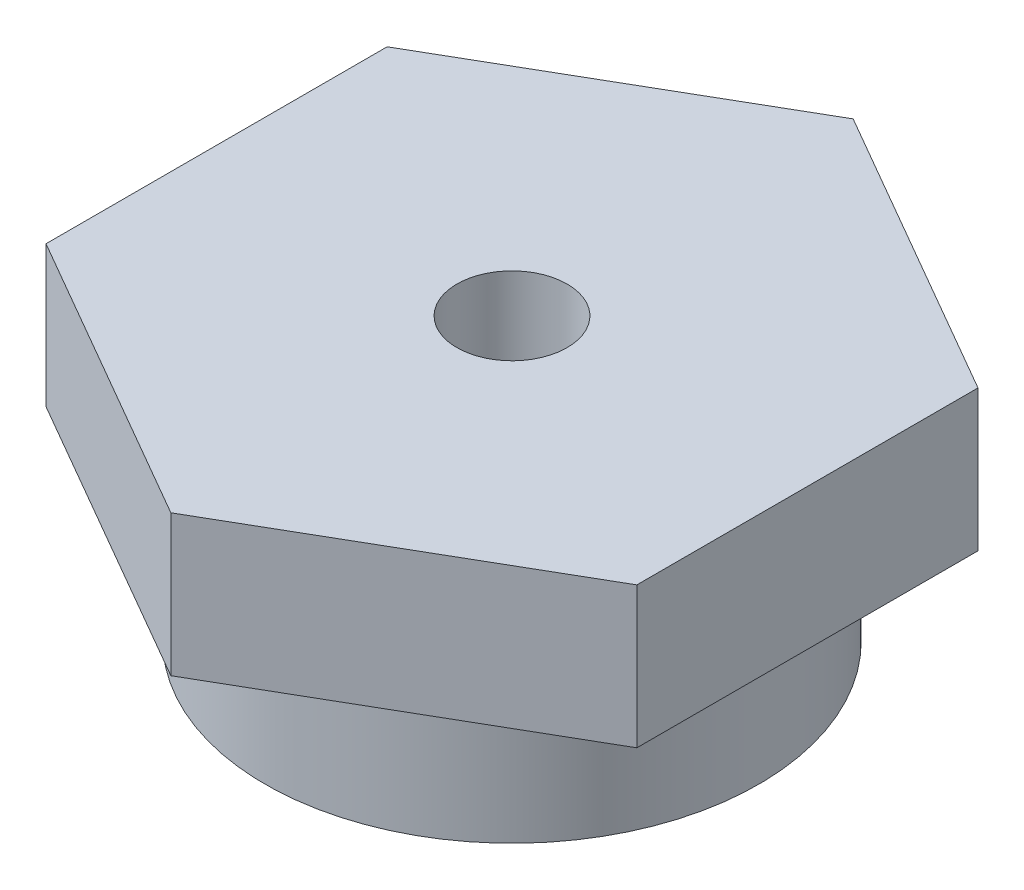
SolidWorks part; units mm, degrees
material "Plain Carbon Steel"
ref_plane "Front Plane" through (0, 0, 0) normal (0, 0, 1) x (1, 0, 0)
ref_plane "Top Plane" through (0, 0, 0) normal (0, 1, 0) x (1, 0, 0)
ref_plane "Right Plane" through (0, 0, 0) normal (1, 0, 0) x (0, 0, -1)
sketch "Hex Profile 67AF" plane through (0, 0, 0) normal (0, 1, 0) x (1, 0, 0)
  line L1 (0, -38.6825) -> (33.5, -19.3412)
  line L2 (33.5, -19.3412) -> (33.5, 19.3412)
  line L3 (33.5, 19.3412) -> (0, 38.6825)
  line L4 (0, 38.6825) -> (-33.5, 19.3412)
  line L5 (-33.5, 19.3412) -> (-33.5, -19.3412)
  line L6 (-33.5, -19.3412) -> (0, -38.6825)
  circle A0 centre (0, 0) radius 33.5 construction
  dimension "D1" = 67
extrude "Hex Body 67AF x16" add sketch "Hex Profile 67AF" along normal blind 16
sketch "Collar Profile Ø56" plane through (0, 0, 0) normal (0, -1, 0) x (1, 0, 0)
  circle A0 centre (0, 0) radius 28
  dimension "D1" = 56
extrude "Collar Ø56 x16" add sketch "Collar Profile Ø56" along normal blind 16
sketch "Bore Profile Ø12.5" plane through (0, -16, 0) normal (0, -1, 0) x (1, 0, 0)
  circle A0 centre (0, 0) radius 6.25
  dimension "D1" = 12.5
extrude "Bore Ø12.5 Through" cut sketch "Bore Profile Ø12.5" against normal through all
